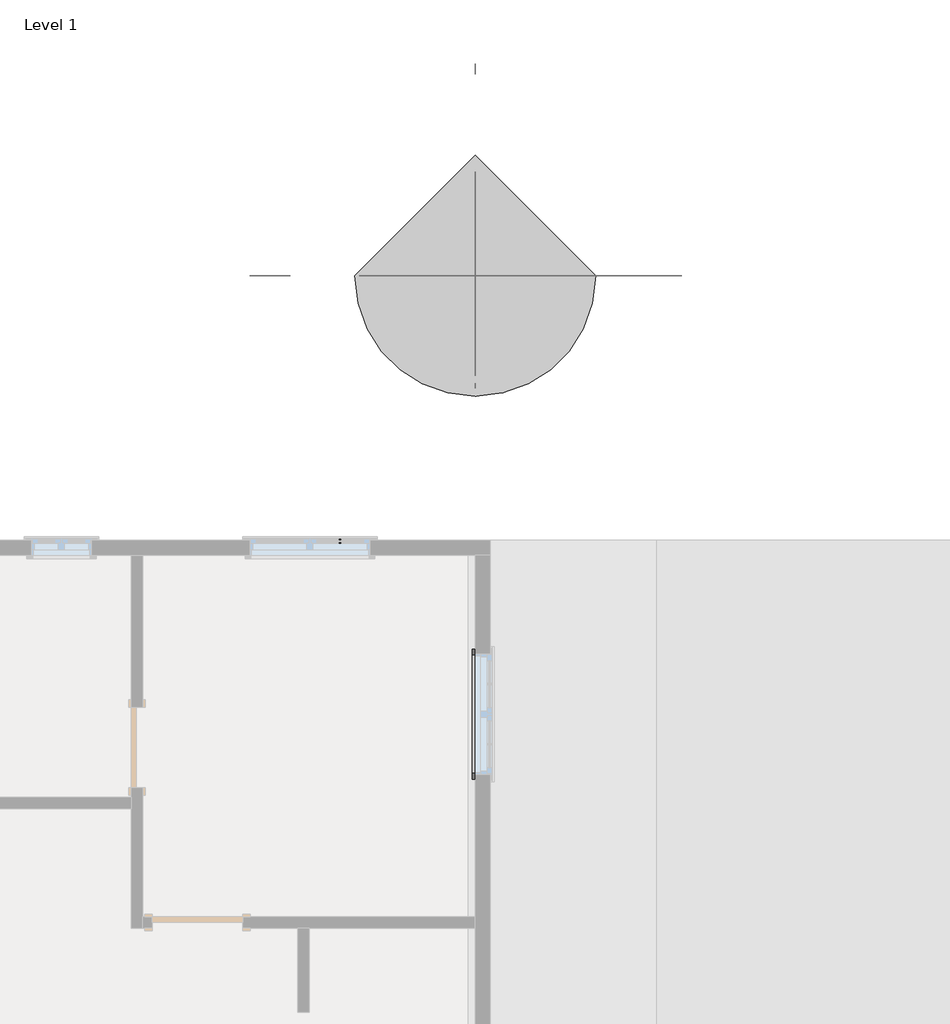
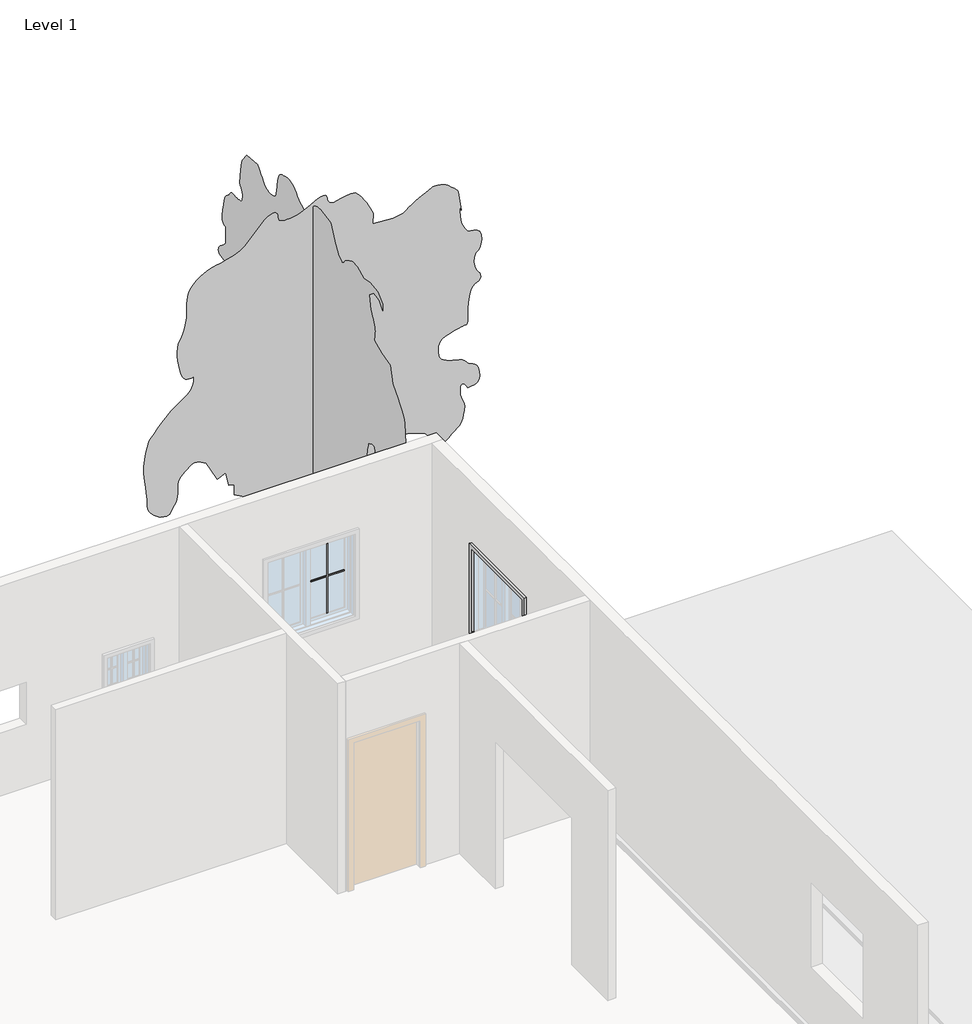
# One storey, part 7 of 7: 2 proxies, 1 geographic element.
"""IFC4 building model written with IfcOpenShell, lengths in millimetres."""

from ifc_helpers import new_model, si_unit, origin, place, context, project, spatial, transform, mapped, element, save
from components import muntin_pattern_2x2_muntin_pattern_2x2_e852a7e4, trim_window_interior_flat_picture_frame_f1e0b15b, rpc_tree_deciduous_golden_chain_18_92130817

model = new_model("IFC4")

# Units and contexts
model_context = context("Model", 3, world=origin())
ifc_project = project(units=[si_unit("LENGTHUNIT", "METRE", prefix="MILLI")], contexts=[model_context])

# Site, building, storey
site = spatial("IfcSite", under=ifc_project)
building = spatial("IfcBuilding", under=site)
storey = spatial("IfcBuildingStorey", under=building, Name="Level 1", Elevation=0.0)

# Proxies
placement = place(None, origin())
muntin_pattern_2x2_muntin_pattern_2x2_shape = muntin_pattern_2x2_muntin_pattern_2x2_e852a7e4(model_context)
element("IfcBuildingElementProxy", 1, Name="Muntin Pattern_2x2 : Muntin Pattern_2x2", ObjectType="Muntin Pattern_2x2 : Muntin Pattern_2x2", at=placement, inside=storey, context=model_context, shape_type="MappedRepresentation", body=[
    mapped(muntin_pattern_2x2_muntin_pattern_2x2_shape, transform((10182.7389317, 13812.8685985, 984.25), x_axis=(-1.0, 0.0, 0.0), y_axis=(0.0, -1.0, 0.0), z_axis=(0.0, 0.0, 1.0))),
])
trim_window_interior_flat_picture_frame_shape = trim_window_interior_flat_picture_frame_f1e0b15b(model_context)
element("IfcBuildingElementProxy", 2, Name="Trim-Window-Interior-Flat : Picture Frame", ObjectType="Trim-Window-Interior-Flat : Picture Frame", at=placement, inside=storey, context=model_context, shape_type="MappedRepresentation", body=[
    mapped(trim_window_interior_flat_picture_frame_shape, transform((11546.4014317, 12069.7935985, 2133.6), x_axis=(0.0, -1.0, 0.0), y_axis=(0.0, 0.0, 1.0), z_axis=(-1.0, 0.0, 0.0))),
])

# Geographic element
rpc_tree_deciduous_golden_chain_18_shape = rpc_tree_deciduous_golden_chain_18_92130817(model_context)
element("IfcGeographicElement", 3, ObjectType="RPC Tree - Deciduous : Golden Chain - 18'", at=placement, inside=storey, context=model_context, shape_type="MappedRepresentation", body=[
    mapped(rpc_tree_deciduous_golden_chain_18_shape, transform((11546.4014317, 16489.3935985, -609.6), x_axis=(1.0, 0.0, 0.0), y_axis=(0.0, 1.0, 0.0), z_axis=(0.0, 0.0, 1.0))),
])

save(model, "model.ifc")

# Revit data of these elements
# Type "Muntin Pattern_2x2 : Muntin Pattern_2x2"
#   Width [instance default] = 4' - 0"
#   Thickness = 0' - 0 1/2"
#   Height [instance default] = 4' - 0"
#   Distance = 0' - 0 3/4"
#   Interior Material [instance default] = none
#   Exterior Material [instance default] = none
#   Default Elevation = 0
# Type "Trim-Window-Interior-Flat : Picture Frame"
#   Trim Thickness_Picture Frame = 0' - 1 1/4"
#   Trim Width = 0' - 2 1/4"
#   Trim Thickness_with Sill = 0' - 0 3/4"
#   Sill Thickness = 0' - 1 1/4"
#   Opening Width [instance default] = 2' - 0"
#   Opening Height [instance default] = 3' - 0"
#   Default Elevation = 4' - 0"
#   Sill = no
#   Picture Frame = yes
#   Trim Material [instance default] = none
# Type "RPC Tree - Deciduous : Golden Chain - 18'"
#   built-in parameter 1005198 = "{2, 15},{39, RPC-16-FXGQ-QK7X-PJ74-6000-ST1L-LVER-AU},{1, 0},{1, 0},{2, 35},{1, 8},{5, Color},{1, 0},{1, 0},{3, 0.8},{3, 0.8},{3, 0.8},{1, 8},{7, BBoxMin},{1, 0},{1, 0},{1, 0},{1, 0},{1, 0},{1, 8},{7, BBoxMax},{1, 0},{1, 0},{1, 0},{1, 0},{1, 0},{2, 11},{9, RPCTypeId},{1, 0},{1, 0},{39, RPC-16-FXGQ-QK7X-PJ74-6000-ST1L-LVER-AU},{1, 6},{14, RPCPlantHeight},{1, 0},{1, 0},{2, 18},{2, 11},{7, keyword},{1, 0},{1, 0},{140, :Geometry:RPC:Golden-chain :Laburnum:Laburnums are very small trees native to southern Europe.  The common cultivar in Canada is 'Watereri'.},{2, 11},{8, category},{1, 0},{1, 0},{16, :Trees [General]},{2, 11},{12, LocalizedUID},{1, 0},{1, 0},{12, Golden-chain},{2, 14},{6, Height},{1, 0},{1, 0},{2, 18},{1, 2},{16, Cast Reflections},{1, 0},{1, 0},{1, 0},{1, 2},{12, Cast Shadows},{1, 0},{1, 0},{1, 1},{1, 2},{9, Lock View},{1, 0},{1, 0},{1, 0},{1, 4},{5, ViewC},{1, 0},{1, 0},{1, 0},{2, 11},{20, AdvancedUIDefinition},{1, 0},{1, 0},{0, },{2, 11},{10, AssetLibID},{1, 0},{1, 0},{36, 4D3F6E72-3F99-4203-98E9-AF80B3C7A7A4},{2, 11},{10, BaseSchema},{1, 0},{1, 0},{9, RPCSchema},{2, 11},{12, ExchangeGUID},{1, 0},{1, 0},{0, },{1, 2},{6, Hidden},{1, 0},{1, 0},{1, 0},{1, 4},{11, RPCCategory},{1, 0},{1, 0},{1, 0},{2, 11},{8, RPCImage},{1, 0},{1, 0},{0, },{1, 4},{13, SchemaVersion},{1, 0},{1, 0},{1, 4},{2, 11},{12, UIDefinition},{1, 0},{1, 0},{0, },{2, 11},{6, UIName},{1, 0},{1, 0},{39, RPC-16-FXGQ-QK7X-PJ74-6000-ST1L-LVER-AU},{2, 11},{11, VersionGUID},{1, 0},{1, 0},{9, RPCSchema},{2, 11},{9, assettype},{1, 0},{1, 0},{11, RPCGeometry},{2, 11},{11, description},{1, 0},{1, 0},{0, },{2, 11},{9, localname},{1, 0},{1, 0},{3, RPC},{2, 11},{9, localtype},{1, 0},{1, 0},{3, RPC},{1, 4},{8, revision},{1, 0},{1, 0},{1, 1},{2, 11},{9, thumbnail},{1, 0},{1, 0},{0, },{1, 4},{7, version},{1, 0},{1, 0},{1, 1},{1, 2},{20, RPC_Cast Reflections},{1, 0},{1, 0},{1, 1},{1, 2},{16, RPC_Cast Shadows},{1, 0},{1, 0},{1, 1},{1, 2},{13, RPC_Lock View},{1, 0},{1, 0},{1, 0},{1, 4},{9, RPC_ViewC},{1, 0},{1, 0},{1, 0},{21, assetlibrary_base.fbx},{1, 5},"
#   built-in parameter 1005195 = "RPC-16-FXGQ-QK7X-PJ74-6000-ST1L-LVER-AU"
#   Type Comments = "Golden Chain"
#   Assembly Code = "G2050500"
#   Height = 18' - 0"
#   Default Elevation = 0
# Element 1 (IfcBuildingElementProxy, "Muntin Pattern_2x2 : Muntin Pattern_2x2")
#   Width = 1' - 6 5/8"
#   Height = 3' - 6 1/2"
#   Interior Material = Wood - Stained
#   Exterior Material = Clad - White
#   Phase Created = New Construction
#   Materials on its faces: "Clad - White", "Wood - Stained"
# Element 2 (IfcBuildingElementProxy, "Trim-Window-Interior-Flat : Picture Frame")
#   Opening Width = 4' - 0"
#   Opening Height = 4' - 0"
#   Trim Material = Wood - Stained
#   Phase Created = New Construction
#   Materials on its faces: "Wood - Stained"
# Element 3 (IfcGeographicElement, "RPC Tree - Deciduous : Golden Chain - 18'")
#   Phase Created = New Construction
# Materials
#   "Clad - White": class "Wood", colour RGB 242 242 238, transparency 0, Cost = 0
#   "Wood - Stained": class "Wood", colour RGB 224 178 126, transparency 0, Cost = 0
